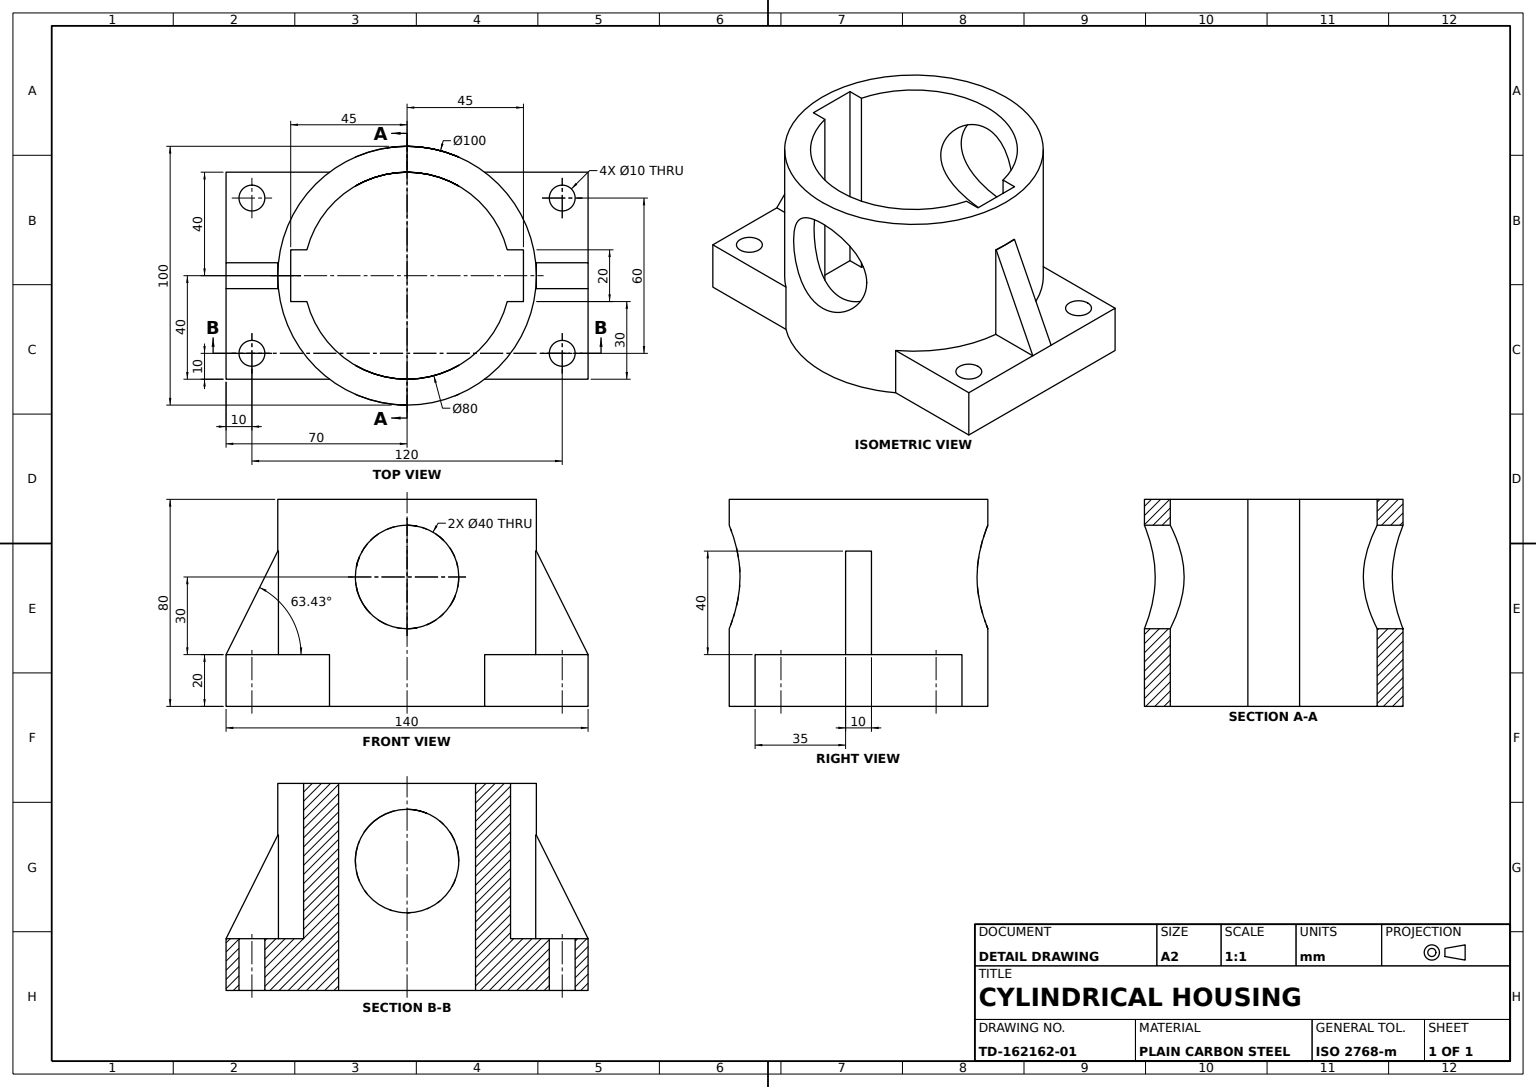
from build123d import *

# Parameters (mm, degrees)
HOUSING_PROFILE_SKETCH_R   = 50
HOUSING_BODY_DEPTH         = 80
BASE_FLANGE_DEPTH          = 20
SUPPORT_RIB_DEPTH          = 5
CROSS_BORE_40_DEPTH        = 118.478919467
CROSS_BORE_40_DEPTH_BACK   = 118.478919467
CROSS_BORE_SKETCH_R        = 20
MOUNTING_HOLES_4X_10_REACH = 106.887
MOUNTING_HOLES_SKETCH_R    = 5


with BuildPart() as part:
    # Housing Profile Sketch → Housing Body (new body)
    with BuildSketch(Plane(origin=(0, 0, 0), x_dir=(1, 0, 0), z_dir=(0, 1, 0))):
        with Locations(Location((0, 0, 0), (0, 0, 270))):
            Circle(HOUSING_PROFILE_SKETCH_R)
        with BuildLine():
            Line((-38.729833462, 10), (-45, 10))
            Line((-45, 10), (-45, -10))
            Line((-45, -10), (-38.729833462, -10))
            ThreePointArc((-38.729833462, -10), (0, -40), (38.729833462, -10))
            Line((38.729833462, -10), (45, -10))
            Line((45, -10), (45, 10))
            Line((45, 10), (38.729833462, 10))
            ThreePointArc((38.729833462, 10), (0, 40), (-38.729833462, 10))
        make_face(mode=Mode.SUBTRACT)
    extrude(amount=HOUSING_BODY_DEPTH)

    # Base Flange Sketch → Base Flange (add)
    with BuildSketch(Plane.XZ):
        with BuildLine():
            Line((30, 40), (70, 40))
            Line((70, 40), (70, -40))
            Line((70, -40), (30, -40))
            ThreePointArc((30, -40), (50, 0), (30, 40))
        make_face()
        with BuildLine():
            Line((-70, -40), (-30, -40))
            ThreePointArc((-30, -40), (-50, 0), (-30, 40))
            Line((-30, 40), (-70, 40))
            Line((-70, 40), (-70, -40))
        make_face()
    extrude(amount=-BASE_FLANGE_DEPTH)

    # Support Rib Sketch → Support Rib (add, symmetric)
    with BuildSketch(Plane.XY):
        Polygon((-50, 60), (-70.009260239, 20), (-50, 20), (-48.125269869, 20), (-48.125269869, 60), align=None)
    support_rib = extrude(amount=SUPPORT_RIB_DEPTH, both=True)

    # Support Rib Mirror: Support Rib across plane
    add(support_rib.mirror(Plane(origin=(0, 0, 0), x_dir=(0, 0, 1), z_dir=(1, 0, 0))))

    # Cross Bore Sketch → Cross Bore Ø40 (cut, two sides: drawn at the far end of the back side and taken through both)
    with BuildSketch(Plane.XY.offset(-CROSS_BORE_40_DEPTH_BACK)):
        with Locations((0, 50)):
            Circle(CROSS_BORE_SKETCH_R)
    extrude(amount=CROSS_BORE_40_DEPTH + CROSS_BORE_40_DEPTH_BACK, mode=Mode.SUBTRACT)

    # Mounting Holes Sketch → Mounting Holes 4xØ10 (cut, up to next)
    with BuildSketch(Plane(origin=(0, 20, 0), x_dir=(1, 0, 0), z_dir=(0, 1, 0)), mode=Mode.PRIVATE) as mounting_holes_4x_10_sk1:
        with Locations(Location((-60, 30, 0), (0, 0, 270))):
            Circle(MOUNTING_HOLES_SKETCH_R)
    mounting_holes_4x_10_tool1 = extrude(mounting_holes_4x_10_sk1.sketch, amount=-MOUNTING_HOLES_4X_10_REACH, mode=Mode.PRIVATE) & part.part
    # Mounting Holes Sketch → Mounting Holes 4xØ10 (cut, up to next)
    with BuildSketch(Plane(origin=(0, 20, 0), x_dir=(1, 0, 0), z_dir=(0, 1, 0)), mode=Mode.PRIVATE) as mounting_holes_4x_10_sk2:
        with Locations(Location((60, 30, 0), (0, 0, 270))):
            Circle(MOUNTING_HOLES_SKETCH_R)
    mounting_holes_4x_10_tool2 = extrude(mounting_holes_4x_10_sk2.sketch, amount=-MOUNTING_HOLES_4X_10_REACH, mode=Mode.PRIVATE) & part.part
    # Mounting Holes Sketch → Mounting Holes 4xØ10 (cut, up to next)
    with BuildSketch(Plane(origin=(0, 20, 0), x_dir=(1, 0, 0), z_dir=(0, 1, 0)), mode=Mode.PRIVATE) as mounting_holes_4x_10_sk3:
        with Locations(Location((60, -30, 0), (0, 0, 270))):
            Circle(MOUNTING_HOLES_SKETCH_R)
    mounting_holes_4x_10_tool3 = extrude(mounting_holes_4x_10_sk3.sketch, amount=-MOUNTING_HOLES_4X_10_REACH, mode=Mode.PRIVATE) & part.part
    # Mounting Holes Sketch → Mounting Holes 4xØ10 (cut, up to next)
    with BuildSketch(Plane(origin=(0, 20, 0), x_dir=(1, 0, 0), z_dir=(0, 1, 0)), mode=Mode.PRIVATE) as mounting_holes_4x_10_sk4:
        with Locations(Location((-60, -30, 0), (0, 0, 270))):
            Circle(MOUNTING_HOLES_SKETCH_R)
    mounting_holes_4x_10_tool4 = extrude(mounting_holes_4x_10_sk4.sketch, amount=-MOUNTING_HOLES_4X_10_REACH, mode=Mode.PRIVATE) & part.part
    add(mounting_holes_4x_10_tool1.solids().sort_by_distance((-60, 20, -30))[0], mode=Mode.SUBTRACT)
    add(mounting_holes_4x_10_tool2.solids().sort_by_distance((60, 20, -30))[0], mode=Mode.SUBTRACT)
    add(mounting_holes_4x_10_tool3.solids().sort_by_distance((60, 20, 30))[0], mode=Mode.SUBTRACT)
    add(mounting_holes_4x_10_tool4.solids().sort_by_distance((-60, 20, 30))[0], mode=Mode.SUBTRACT)


solid = part.part
